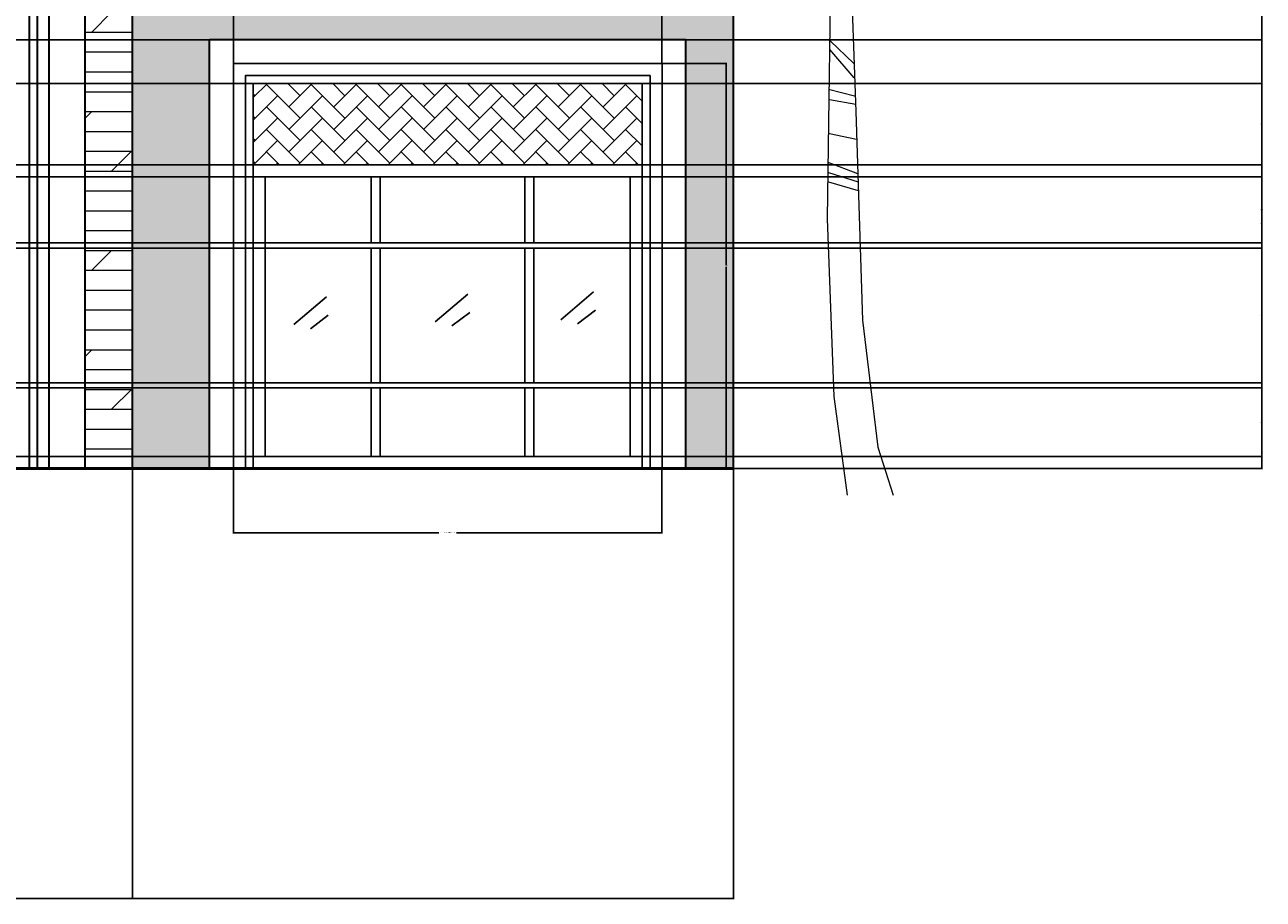
# Model space of a CAD drawing. Units: inches. Extents: x -13 to 630, y -103 to 275.
# Tile 8 of 9: x 318 to 630, y -103 to 117. Entities that reach past the tile are written whole.
import ezdxf

# ---------------------------------------------------------------- set-up
doc = ezdxf.new("R2010")
doc.units = ezdxf.units.IN
doc.header["$MEASUREMENT"] = 0
for name, color, linetype, lineweight in [('A-ANNO-DIMS', 2, 'Continuous', 18), ('A-ELEV', 7, 'Continuous', 35), ('A-ELEV-GRND', 7, 'Continuous', 50), ('A-ELEV-PATT', 8, 'Continuous', 13), ('A-GLAZ', 4, 'Continuous', 25), ('L-PLNT', 3, 'Continuous', 13)]:
    doc.layers.add(name, color=color, linetype=linetype, lineweight=lineweight)
doc.styles.get("Standard").update_dxf_attribs({"font": 'arial.ttf'})
doc.dimstyles.get("Standard").update_dxf_attribs({"dimtxt": 0.18, "dimasz": 0.18, "dimexe": 0.18, "dimexo": 0.0625, "dimgap": 0.09, "dimtad": 0, "dimtih": 1, "dimtoh": 1, "dimdec": 4, "dimzin": 0, "dimdsep": 46, "dimtxsty": 'Standard', "dimcen": 0.09, "dimadec": 0, "dimazin": 0, "dimtfac": 1, "dimtdec": 4, "dimtofl": 0, "dimtmove": 0, "dimatfit": 3, "dimfxl": 1, "dimtolj": 1, "dimtzin": 0, "dimarcsym": 0})

# ---------------------------------------------------------------- blocks, each defined once
blk = doc.blocks.new('*U2')
for p, q in [((-5.567, 196.707), (-4.987, 201.167)), ((-4.407, 195.716), (-3.247, 200.672)), ((-6.727, 197.202), (-11.366, 197.45)), ((-7.5, 199.68), (-7.5, 197.946)), ((-2.474, 193.733), (-1.315, 199.433)), ((-1.121, 190.759), (0.232, 196.955)), ((9.317, 191.255), (10.283, 196.955)), ((11.829, 192.99), (13.182, 197.45)), ((13.956, 194.229), (14.729, 196.955)), ((15.116, 194.477), (17.822, 198.689)), ((18.015, 195.716), (20.914, 198.689)), ((21.301, 196.459), (22.847, 198.441)), ((22.074, 196.707), (23.427, 195.716)), ((23.234, 196.707), (23.62, 197.698)), ((-15.232, 191.255), (-20.644, 193.981)), ((-3.441, 194.477), (-10.013, 195.716)), ((-1.894, 192.494), (-9.24, 193.733)), ((0.038, 188.281), (1.778, 193.981)), ((5.837, 187.786), (7.577, 194.229)), ((14.536, 193.981), (17.242, 191.255)), ((16.082, 194.972), (17.822, 192.494)), ((18.015, 195.468), (18.981, 192.494)), ((19.368, 196.459), (19.948, 193.733)), ((20.914, 196.459), (21.301, 194.972)), ((-29.729, 190.759), (-31.469, 191.255)), ((-30.309, 190.512), (-30.695, 189.025)), ((-25.283, 191.751), (-29.342, 192.246)), ((-28.763, 190.759), (-28.763, 188.281)), ((-26.443, 191.503), (-26.636, 186.051)), ((-20.064, 191.751), (-25.863, 193.238)), ((-23.737, 191.751), (-24.51, 185.06)), ((-21.031, 191.998), (-21.804, 183.325)), ((-17.551, 191.503), (-20.451, 181.343)), ((-14.265, 190.759), (-18.131, 182.086)), ((-9.433, 189.025), (-15.618, 193.238)), ((-0.541, 189.52), (-7.307, 192.494)), ((1.005, 185.803), (2.358, 190.759)), ((4.098, 185.06), (4.678, 190.512)), ((8.544, 190.512), (13.763, 189.52)), ((11.25, 192.494), (15.889, 190.512)), ((-11.753, 189.768), (-15.425, 182.83)), ((-8.08, 188.034), (-12.912, 182.83)), ((-6.147, 186.299), (-9.24, 190.264)), ((-5.76, 190.016), (0.618, 185.308)), ((-5.76, 188.034), (-1.508, 182.582)), ((6.997, 188.529), (12.216, 187.786)), ((9.51, 184.317), (15.502, 188.034)), ((15.695, 186.299), (19.368, 188.777)), ((19.368, 187.29), (26.133, 189.768)), ((23.814, 187.29), (26.907, 181.343)), ((24.78, 187.538), (31.546, 188.777)), ((26.133, 187.29), (29.419, 181.838)), ((28.066, 187.29), (30.966, 182.582)), ((29.999, 186.795), (33.092, 187.29)), ((-4.987, 185.803), (-10.979, 182.086)), ((-2.668, 185.803), (1.198, 181.343)), ((1.005, 182.582), (2.938, 186.547)), ((4.871, 186.051), (10.09, 186.547)), ((4.871, 181.591), (8.544, 184.812)), ((11.25, 184.812), (17.628, 180.352)), ((14.536, 185.803), (19.948, 180.847)), ((17.242, 186.547), (23.041, 180.599)), ((20.721, 187.042), (25.167, 181.343)), ((29.806, 186.795), (32.319, 183.078)), ((32.512, 186.299), (35.218, 186.299)), ((33.479, 186.051), (34.445, 182.83)), ((35.605, 185.556), (37.151, 185.308)), ((35.798, 185.308), (36.958, 181.591)), ((38.118, 184.317), (38.504, 181.838)), ((-3.247, 183.821), (-8.08, 181.838)), ((-1.315, 181.591), (-5.374, 181.095)), ((2.938, 182.582), (6.61, 183.821)), ((5.644, 181.838), (13.569, 178.865)), ((7.77, 183.325), (16.082, 179.856)), ((39.857, 182.83), (40.244, 181.591)), ((-15.618, 179.36), (-20.644, 178.617)), ((-17.358, 178.617), (-13.299, 173.661)), ((-15.038, 179.36), (-10.786, 174.404)), ((-12.332, 180.104), (-9.433, 175.643)), ((-10.206, 180.104), (-8.08, 175.891)), ((-8.273, 180.104), (-6.147, 176.635)), ((-6.34, 179.608), (-4.6, 177.13)), ((-4.021, 179.36), (-2.861, 177.378)), ((-0.348, 180.352), (-1.894, 180.104)), ((4.098, 180.847), (8.35, 179.608)), ((6.224, 178.121), (8.157, 175.148)), ((7.384, 178.369), (10.476, 179.36)), ((8.157, 178.121), (10.476, 172.422)), ((11.829, 177.874), (18.015, 179.113)), ((18.015, 177.13), (26.133, 179.113)), ((-25.09, 175.148), (-28.376, 174.404)), ((-21.031, 177.626), (-24.897, 176.387)), ((-24.317, 175.891), (-18.711, 168.457)), ((-22.191, 176.635), (-16.391, 169.448)), ((-20.064, 177.626), (-15.812, 172.67)), ((-4.214, 175.148), (-14.072, 170.935)), ((-1.701, 176.882), (-8.66, 175.396)), ((-4.6, 174.9), (-4.021, 166.722)), ((-2.668, 176.387), (-2.376, 170.594)), ((-0.928, 176.882), (-1.508, 173.909)), ((2.551, 175.891), (-0.928, 171.431)), ((1.585, 177.13), (0.038, 174.652)), ((1.585, 177.13), (6.61, 176.139)), ((2.938, 175.891), (8.737, 173.413)), ((10.476, 177.874), (12.796, 169.696)), ((13.182, 177.874), (14.729, 166.97)), ((15.889, 177.13), (16.855, 164.492)), ((18.981, 175.891), (19.561, 163.005)), ((20.914, 175.891), (30.966, 176.635)), ((21.688, 175.396), (22.074, 161.518)), ((-28.956, 172.174), (-32.435, 170.192)), ((-27.409, 173.413), (-30.695, 172.67)), ((-27.989, 172.422), (-26.056, 166.227)), ((-26.829, 173.661), (-23.544, 167.218)), ((-25.476, 174.652), (-21.224, 167.466)), ((-8.466, 171.678), (-16.585, 167.713)), ((-6.92, 172.917), (-5.374, 163.253)), ((3.711, 174.404), (-0.541, 167.961)), ((5.257, 171.926), (-0.155, 163.005)), ((4.291, 173.909), (12.216, 168.953)), ((23.814, 174.404), (25.554, 160.279)), ((25.554, 173.661), (33.285, 173.661)), ((26.52, 173.165), (28.066, 159.784)), ((28.839, 172.174), (36.378, 170.687)), ((29.226, 171.926), (30.966, 158.545)), ((-31.082, 169.944), (-32.435, 169.2)), ((-31.662, 168.705), (-31.082, 165.483)), ((-29.922, 170.687), (-27.989, 165.235)), ((-8.853, 170.935), (-7.113, 160.527)), ((7.384, 168.705), (0.812, 157.553)), ((6.417, 170.439), (14.729, 164.492)), ((30.966, 170.687), (38.891, 167.713)), ((32.126, 169.696), (32.512, 158.545)), ((34.058, 168.705), (34.445, 158.545)), ((-32.628, 167.961), (-33.208, 167.961)), ((-32.628, 167.713), (-32.435, 165.979)), ((-12.139, 167.961), (-19.098, 162.014)), ((-12.719, 166.722), (-9.046, 154.828)), ((-10.979, 168.457), (-7.887, 157.801)), ((8.544, 165.979), (16.662, 160.527)), ((35.412, 167.713), (41.404, 164.988)), ((36.378, 166.474), (35.605, 158.792)), ((-14.265, 164.244), (-19.678, 158.049)), ((-14.265, 163.749), (-10.786, 154.828)), ((9.317, 164.244), (2.358, 154.332)), ((10.09, 162.51), (17.435, 157.058)), ((37.731, 165.235), (36.958, 159.288)), ((37.924, 165.235), (41.404, 163.749)), ((38.504, 164.492), (38.504, 159.536)), ((39.664, 163.253), (42.37, 161.766)), ((39.857, 162.757), (39.857, 160.031)), ((-16.005, 160.031), (-19.484, 154.084)), ((-15.618, 160.775), (-12.332, 154.332)), ((10.863, 159.784), (4.484, 152.35)), ((40.824, 161.766), (41.21, 160.031)), ((41.21, 161.518), (42.757, 160.279)), ((-16.585, 158.545), (-13.106, 152.35)), ((11.443, 157.553), (16.855, 154.332)), ((-18.131, 153.589), (-19.484, 151.606)), ((-17.358, 155.819), (-14.845, 151.358)), ((11.829, 155.075), (6.804, 150.119)), ((12.216, 153.093), (16.082, 151.606)), ((-17.938, 152.597), (-16.972, 151.111)), ((12.603, 151.111), (8.544, 148.385)), ((12.603, 149.872), (15.116, 149.128)), ((12.216, 148.137), (10.09, 147.393)), ((12.409, 146.898), (13.763, 146.402)), ((12.409, 145.659), (11.056, 145.659)), ((-4.081, 140.645), (0.753, 138.261)), ((-4.081, 137.547), (0.753, 135.163)), ((-4.081, 129.205), (1.124, 126.821)), ((-4.081, 127.298), (1.31, 123.246)), ((-4.081, 121.578), (1.31, 120.863)), ((-4.267, 114.428), (1.682, 108.708)), ((-4.453, 112.283), (1.682, 105.133)), ((-4.639, 102.273), (1.868, 100.604)), ((-4.453, 99.651), (2.24, 98.459)), ((-4.453, 91.071), (2.426, 89.641)), ((-4.825, 83.921), (2.612, 81.061)), ((-4.639, 81.299), (2.797, 78.916)), ((-4.639, 78.916), (2.797, 76.771))]:
    blk.add_line(p, q)
for points in [[(-2.363, 170.553), (-3.88, 148.505), (-4.988, 69.634), (-3.325, 24.869), (0, 0)], [(-0.116, 162.848), (0.554, 143.532), (2.217, 96.635), (3.88, 44.054), (7.76, 12.079), (11.64, 0)]]:
    blk.add_lwpolyline(points)
for centre, radius, start, end in [((-18.427, 181.448), 19.715, 350.285, 64.11229), ((25.595, 171.567), 25.395, 91.40319, 163.882), ((-21.738, 166.094), 25.899, 27.67115, 112.5305), ((23.687, 155.341), 32.188, 56.19272, 134.3213), ((-9.259, 151.732), 28.386, 68.38311, 147.5322), ((14.394, 148.393), 32.752, 113.7592, 177.4133), ((5.828, 132.718), 45.639, 35.98777, 95.82273), ((-32.8, 147.923), 45.309, 356.1943, 41.37848)]:
    blk.add_arc(centre, radius, start, end)
blk = doc.blocks.new('WIN-GROUND')
for points in [[(0, 0), (0, 102), (108, 102), (108, 0)], [(3, 0), (3, 99), (105, 99), (105, 0)], [(5, 0), (5, 97), (103, 97), (103, 0)], [(34.74, 56.82), (34.74, 73.49), (37, 73.49), (37, 56.82)], [(73.43, 56.82), (73.43, 73.49), (75.7, 73.49), (75.7, 56.82)], [(34.74, 55.51), (8, 55.51), (8, 56.82), (34.74, 56.82)], [(37, 56.82), (73.43, 56.82)], [(75.7, 56.82), (100, 56.82), (100, 55.51), (75.7, 55.51)], [(34.74, 21.58), (34.74, 55.51)], [(37, 55.51), (37, 21.58)], [(73.43, 55.51), (37, 55.51)], [(73.43, 21.58), (73.43, 55.51)], [(75.7, 55.51), (75.7, 21.58)], [(34.74, 20.27), (8, 20.27), (8, 21.58), (34.74, 21.58)], [(37, 20.27), (37, 3), (34.74, 3), (34.74, 20.27)], [(37, 21.58), (73.43, 21.58)], [(73.43, 20.27), (37, 20.27)], [(75.7, 20.27), (75.7, 3), (73.43, 3), (73.43, 20.27)], [(75.7, 21.58), (100, 21.58), (100, 20.27), (75.7, 20.27)]]:
    blk.add_lwpolyline(points)
for points in [[(5, 97), (103, 97), (103, 76.49), (5, 76.49)], [(5, 76.49), (103, 76.49), (103, 0), (5, 0)], [(8, 73.49), (100, 73.49), (100, 3), (8, 3)]]:
    blk.add_lwpolyline(points, close=True)
blk = doc.blocks.new('GLAZ-MARK')
for p, q in [((0, 1.02), (8.26, 8.03)), ((4.19, 0), (8.71, 3.39))]:
    blk.add_line(p, q)
blk = doc.blocks.new('*D5')
at = {"layer": 'A-ANNO-DIMS', "color": 0, "lineweight": -2, "transparency": 16777216}
for p, q in [((370.71, 5.02), (370.71, -11.3)), ((478.71, 5.02), (478.71, -11.3)), ((370.89, -11.12), (422.47, -11.12)), ((478.53, -11.12), (426.96, -11.12))]:
    blk.add_line(p, q, dxfattribs=at)
at = {"layer": 'A-ANNO-DIMS', "color": 0, "transparency": 16777216}
for points in [[(370.89, -11.09), (370.89, -11.15), (370.71, -11.12)], [(478.53, -11.09), (478.53, -11.15), (478.71, -11.12)]]:
    blk.add_solid(points, dxfattribs=at)
at = {"layer": 'Defpoints', "color": 0, "transparency": 16777216}
for p in [(370.71, 5.08), (478.71, 5.08), (478.71, -11.12)]:
    blk.add_point(p, dxfattribs=at)
at = {"layer": 'A-ANNO-DIMS', "color": 0, "transparency": 16777216, "insert": (424.71, -11.12), "char_height": 0.18, "attachment_point": 5}
blk.add_mtext('\\A1;GROUND FLOOR WINDOW 108 TYP.', dxfattribs=at)
blk = doc.blocks.new('*D6')
at = {"layer": 'A-ANNO-DIMS', "color": 0, "lineweight": -2, "transparency": 16777216}
for p, q in [((478.77, 107.08), (495.09, 107.08)), ((494.91, 106.9), (494.91, 56.26)), ((494.91, 5.26), (494.91, 55.9)), ((478.77, 5.08), (495.09, 5.08))]:
    blk.add_line(p, q, dxfattribs=at)
at = {"layer": 'A-ANNO-DIMS', "color": 0, "transparency": 16777216}
for points in [[(494.88, 106.9), (494.94, 106.9), (494.91, 107.08)], [(494.88, 5.26), (494.94, 5.26), (494.91, 5.08)]]:
    blk.add_solid(points, dxfattribs=at)
at = {"layer": 'Defpoints', "color": 0, "transparency": 16777216}
for p in [(478.71, 107.08), (494.91, 107.08), (478.71, 5.08)]:
    blk.add_point(p, dxfattribs=at)
at = {"layer": 'A-ANNO-DIMS', "color": 0, "transparency": 16777216, "insert": (494.91, 56.08), "char_height": 0.18, "attachment_point": 5}
blk.add_mtext('\\A1;102 TYP.', dxfattribs=at)
blk = doc.blocks.new('*D9')
at = {"layer": 'A-ANNO-DIMS', "color": 0, "lineweight": -2, "transparency": 16777216}
for p, q in [((345.31, 5.14), (345.31, 275.01)), ((345.49, 274.83), (357.54, 274.83)), ((370.53, 274.83), (358.47, 274.83)), ((370.71, 5.14), (370.71, 275.01))]:
    blk.add_line(p, q, dxfattribs=at)
at = {"layer": 'A-ANNO-DIMS', "color": 0, "transparency": 16777216}
for points in [[(345.49, 274.86), (345.49, 274.8), (345.31, 274.83)], [(370.53, 274.86), (370.53, 274.8), (370.71, 274.83)]]:
    blk.add_solid(points, dxfattribs=at)
at = {"layer": 'Defpoints', "color": 0, "transparency": 16777216}
for p in [(370.71, 274.83), (345.31, 5.08), (370.71, 5.08)]:
    blk.add_point(p, dxfattribs=at)
at = {"layer": 'A-ANNO-DIMS', "color": 0, "transparency": 16777216, "insert": (358.01, 274.83), "char_height": 0.18, "attachment_point": 5}
blk.add_mtext('\\A1;25.406', dxfattribs=at)
blk = doc.blocks.new('*D10')
at = {"layer": 'A-ANNO-DIMS', "color": 0, "lineweight": -2, "transparency": 16777216}
for p, q in [((478.71, 107.14), (478.71, 275.01)), ((478.89, 274.83), (487.5, 274.83)), ((496.53, 274.83), (487.92, 274.83)), ((496.71, 125.14), (496.71, 275.01))]:
    blk.add_line(p, q, dxfattribs=at)
at = {"layer": 'A-ANNO-DIMS', "color": 0, "transparency": 16777216}
for points in [[(478.89, 274.86), (478.89, 274.8), (478.71, 274.83)], [(496.53, 274.86), (496.53, 274.8), (496.71, 274.83)]]:
    blk.add_solid(points, dxfattribs=at)
at = {"layer": 'Defpoints', "color": 0, "transparency": 16777216}
for p in [(496.71, 274.83), (496.71, 125.08), (478.71, 107.08)]:
    blk.add_point(p, dxfattribs=at)
at = {"layer": 'A-ANNO-DIMS', "color": 0, "transparency": 16777216, "insert": (487.71, 274.83), "char_height": 0.18, "attachment_point": 5}
blk.add_mtext('\\A1;18', dxfattribs=at)
blk = doc.blocks.new('*D11')
at = {"layer": 'A-ANNO-DIMS', "color": 0, "lineweight": -2, "transparency": 16777216}
for p, q in [((16.71, 5.02), (16.71, -103.45)), ((496.71, 5.02), (496.71, -103.45)), ((16.89, -103.27), (256.42, -103.27)), ((496.53, -103.27), (257, -103.27))]:
    blk.add_line(p, q, dxfattribs=at)
at = {"layer": 'A-ANNO-DIMS', "color": 0, "transparency": 16777216}
for points in [[(16.89, -103.24), (16.89, -103.3), (16.71, -103.27)], [(496.53, -103.24), (496.53, -103.3), (496.71, -103.27)]]:
    blk.add_solid(points, dxfattribs=at)
at = {"layer": 'Defpoints', "color": 0, "transparency": 16777216}
for p in [(16.71, 5.08), (496.71, 5.08), (496.71, -103.27)]:
    blk.add_point(p, dxfattribs=at)
at = {"layer": 'A-ANNO-DIMS', "color": 0, "transparency": 16777216, "insert": (256.71, -103.27), "char_height": 0.18, "attachment_point": 5}
blk.add_mtext('\\A1;480', dxfattribs=at)
blk = doc.blocks.new('*D13')
at = {"layer": 'A-ANNO-DIMS', "color": 0, "lineweight": -2, "transparency": 16777216}
for p, q in [((345.37, 245.08), (630.03, 245.08)), ((629.85, 244.9), (629.85, 125.26)), ((629.85, 5.26), (629.85, 124.9)), ((496.77, 5.08), (630.03, 5.08))]:
    blk.add_line(p, q, dxfattribs=at)
at = {"layer": 'A-ANNO-DIMS', "color": 0, "transparency": 16777216}
for points in [[(629.82, 244.9), (629.88, 244.9), (629.85, 245.08)], [(629.82, 5.26), (629.88, 5.26), (629.85, 5.08)]]:
    blk.add_solid(points, dxfattribs=at)
at = {"layer": 'Defpoints', "color": 0, "transparency": 16777216}
for p in [(345.31, 245.08), (629.85, 245.08), (496.71, 5.08)]:
    blk.add_point(p, dxfattribs=at)
at = {"layer": 'A-ANNO-DIMS', "color": 0, "transparency": 16777216, "insert": (629.85, 125.08), "char_height": 0.18, "attachment_point": 5}
blk.add_mtext('\\A1;240', dxfattribs=at)
blk = doc.blocks.new('*D26')
at = {"layer": 'A-ANNO-DIMS', "color": 0, "lineweight": -2, "transparency": 16777216}
for p, q in [((302.53, 5.02), (302.53, -103.45)), ((345.31, 5.02), (345.31, -103.45)), ((302.71, -103.27), (323.52, -103.27)), ((345.13, -103.27), (324.31, -103.27))]:
    blk.add_line(p, q, dxfattribs=at)
at = {"layer": 'A-ANNO-DIMS', "color": 0, "transparency": 16777216}
for points in [[(302.71, -103.24), (302.71, -103.3), (302.53, -103.27)], [(345.13, -103.24), (345.13, -103.3), (345.31, -103.27)]]:
    blk.add_solid(points, dxfattribs=at)
at = {"layer": 'Defpoints', "color": 0, "transparency": 16777216}
for p in [(302.53, 5.08), (345.31, 5.08), (345.31, -103.27)]:
    blk.add_point(p, dxfattribs=at)
at = {"layer": 'A-ANNO-DIMS', "color": 0, "transparency": 16777216, "insert": (323.92, -103.27), "char_height": 0.18, "attachment_point": 5}
blk.add_mtext('\\A1;42.78', dxfattribs=at)
blk = doc.blocks.new('*D28')
at = {"layer": 'A-ANNO-DIMS', "color": 0, "lineweight": -2, "transparency": 16777216}
for p, q in [((302.59, 128.66), (630.03, 128.66)), ((629.85, 128.48), (629.85, 67.05)), ((629.85, 5.26), (629.85, 66.69)), ((302.59, 5.08), (630.03, 5.08))]:
    blk.add_line(p, q, dxfattribs=at)
at = {"layer": 'A-ANNO-DIMS', "color": 0, "transparency": 16777216}
for points in [[(629.82, 128.48), (629.88, 128.48), (629.85, 128.66)], [(629.82, 5.26), (629.88, 5.26), (629.85, 5.08)]]:
    blk.add_solid(points, dxfattribs=at)
at = {"layer": 'Defpoints', "color": 0, "transparency": 16777216}
for p in [(302.53, 128.66), (629.85, 128.66), (302.53, 5.08)]:
    blk.add_point(p, dxfattribs=at)
at = {"layer": 'A-ANNO-DIMS', "color": 0, "transparency": 16777216, "insert": (629.85, 66.87), "char_height": 0.18, "attachment_point": 5}
blk.add_mtext('\\A1;123.57', dxfattribs=at)
blk = doc.blocks.new('*D78')
at = {"layer": 'A-ANNO-DIMS', "color": 0, "lineweight": -2, "transparency": 16777216}
for p, q in [((134.77, 8.08), (630.03, 8.08)), ((629.85, 7.9), (629.85, 6.76)), ((629.85, 5.26), (629.85, 6.4)), ((137.77, 5.08), (630.03, 5.08))]:
    blk.add_line(p, q, dxfattribs=at)
at = {"layer": 'A-ANNO-DIMS', "color": 0, "transparency": 16777216}
for points in [[(629.82, 7.9), (629.88, 7.9), (629.85, 8.08)], [(629.82, 5.26), (629.88, 5.26), (629.85, 5.08)]]:
    blk.add_solid(points, dxfattribs=at)
at = {"layer": 'Defpoints', "color": 0, "transparency": 16777216}
for p in [(134.71, 8.08), (629.85, 8.08), (137.71, 5.08)]:
    blk.add_point(p, dxfattribs=at)
at = {"layer": 'A-ANNO-DIMS', "color": 0, "transparency": 16777216, "insert": (629.85, 6.58), "char_height": 0.18, "attachment_point": 5}
blk.add_mtext('\\A1;3', dxfattribs=at)
blk = doc.blocks.new('*D79')
at = {"layer": 'A-ANNO-DIMS', "color": 0, "lineweight": -2, "transparency": 16777216}
for p, q in [((134.77, 25.35), (630.03, 25.35)), ((629.85, 25.17), (629.85, 16.9)), ((629.85, 8.26), (629.85, 16.53)), ((134.77, 8.08), (630.03, 8.08))]:
    blk.add_line(p, q, dxfattribs=at)
at = {"layer": 'A-ANNO-DIMS', "color": 0, "transparency": 16777216}
for points in [[(629.82, 25.17), (629.88, 25.17), (629.85, 25.35)], [(629.82, 8.26), (629.88, 8.26), (629.85, 8.08)]]:
    blk.add_solid(points, dxfattribs=at)
at = {"layer": 'Defpoints', "color": 0, "transparency": 16777216}
for p in [(134.71, 25.35), (629.85, 25.35), (134.71, 8.08)]:
    blk.add_point(p, dxfattribs=at)
at = {"layer": 'A-ANNO-DIMS', "color": 0, "transparency": 16777216, "insert": (629.85, 16.72), "char_height": 0.18, "attachment_point": 5}
blk.add_mtext('\\A1;17.27', dxfattribs=at)
blk = doc.blocks.new('*D80')
at = {"layer": 'A-ANNO-DIMS', "color": 0, "lineweight": -2, "transparency": 16777216}
for p, q in [((134.77, 26.66), (630.03, 26.66)), ((134.77, 25.35), (630.03, 25.35)), ((629.85, 26.48), (629.85, 26.19)), ((629.85, 25.53), (629.85, 25.82))]:
    blk.add_line(p, q, dxfattribs=at)
at = {"layer": 'A-ANNO-DIMS', "color": 0, "transparency": 16777216}
for points in [[(629.82, 26.48), (629.88, 26.48), (629.85, 26.66)], [(629.82, 25.53), (629.88, 25.53), (629.85, 25.35)]]:
    blk.add_solid(points, dxfattribs=at)
at = {"layer": 'Defpoints', "color": 0, "transparency": 16777216}
for p in [(134.71, 26.66), (134.71, 25.35), (629.85, 26.66)]:
    blk.add_point(p, dxfattribs=at)
at = {"layer": 'A-ANNO-DIMS', "color": 0, "transparency": 16777216, "insert": (629.85, 26), "char_height": 0.18, "attachment_point": 5}
blk.add_mtext('\\A1;1.31', dxfattribs=at)
blk = doc.blocks.new('*D81')
at = {"layer": 'A-ANNO-DIMS', "color": 0, "lineweight": -2, "transparency": 16777216}
for p, q in [((134.77, 60.6), (630.03, 60.6)), ((629.85, 60.42), (629.85, 43.81)), ((629.85, 26.84), (629.85, 43.44)), ((134.77, 26.66), (630.03, 26.66))]:
    blk.add_line(p, q, dxfattribs=at)
at = {"layer": 'A-ANNO-DIMS', "color": 0, "transparency": 16777216}
for points in [[(629.82, 60.42), (629.88, 60.42), (629.85, 60.6)], [(629.82, 26.84), (629.88, 26.84), (629.85, 26.66)]]:
    blk.add_solid(points, dxfattribs=at)
at = {"layer": 'Defpoints', "color": 0, "transparency": 16777216}
for p in [(134.71, 60.6), (629.85, 60.6), (134.71, 26.66)]:
    blk.add_point(p, dxfattribs=at)
at = {"layer": 'A-ANNO-DIMS', "color": 0, "transparency": 16777216, "insert": (629.85, 43.63), "char_height": 0.18, "attachment_point": 5}
blk.add_mtext('\\A1;33.94', dxfattribs=at)
blk = doc.blocks.new('*D82')
at = {"layer": 'A-ANNO-DIMS', "color": 0, "lineweight": -2, "transparency": 16777216}
for p, q in [((134.77, 61.9), (630.03, 61.9)), ((134.77, 60.6), (630.03, 60.6)), ((629.85, 61.72), (629.85, 61.43)), ((629.85, 60.78), (629.85, 61.07))]:
    blk.add_line(p, q, dxfattribs=at)
at = {"layer": 'A-ANNO-DIMS', "color": 0, "transparency": 16777216}
for points in [[(629.82, 61.72), (629.88, 61.72), (629.85, 61.9)], [(629.82, 60.78), (629.88, 60.78), (629.85, 60.6)]]:
    blk.add_solid(points, dxfattribs=at)
at = {"layer": 'Defpoints', "color": 0, "transparency": 16777216}
for p in [(134.71, 61.9), (134.71, 60.6), (629.85, 61.9)]:
    blk.add_point(p, dxfattribs=at)
at = {"layer": 'A-ANNO-DIMS', "color": 0, "transparency": 16777216, "insert": (629.85, 61.25), "char_height": 0.18, "attachment_point": 5}
blk.add_mtext('\\A1;1.31', dxfattribs=at)
blk = doc.blocks.new('*D83')
at = {"layer": 'A-ANNO-DIMS', "color": 0, "lineweight": -2, "transparency": 16777216}
for p, q in [((134.77, 78.57), (630.03, 78.57)), ((629.85, 78.39), (629.85, 70.42)), ((629.85, 62.08), (629.85, 70.05)), ((134.77, 61.9), (630.03, 61.9))]:
    blk.add_line(p, q, dxfattribs=at)
at = {"layer": 'A-ANNO-DIMS', "color": 0, "transparency": 16777216}
for points in [[(629.82, 78.39), (629.88, 78.39), (629.85, 78.57)], [(629.82, 62.08), (629.88, 62.08), (629.85, 61.9)]]:
    blk.add_solid(points, dxfattribs=at)
at = {"layer": 'Defpoints', "color": 0, "transparency": 16777216}
for p in [(134.71, 78.57), (629.85, 78.57), (134.71, 61.9)]:
    blk.add_point(p, dxfattribs=at)
at = {"layer": 'A-ANNO-DIMS', "color": 0, "transparency": 16777216, "insert": (629.85, 70.24), "char_height": 0.18, "attachment_point": 5}
blk.add_mtext('\\A1;16.67', dxfattribs=at)
blk = doc.blocks.new('*D84')
at = {"layer": 'A-ANNO-DIMS', "color": 0, "lineweight": -2, "transparency": 16777216}
for p, q in [((137.77, 81.57), (630.03, 81.57)), ((629.85, 81.39), (629.85, 80.25)), ((134.77, 78.57), (630.03, 78.57)), ((629.85, 78.75), (629.85, 79.89))]:
    blk.add_line(p, q, dxfattribs=at)
at = {"layer": 'A-ANNO-DIMS', "color": 0, "transparency": 16777216}
for points in [[(629.82, 81.39), (629.88, 81.39), (629.85, 81.57)], [(629.82, 78.75), (629.88, 78.75), (629.85, 78.57)]]:
    blk.add_solid(points, dxfattribs=at)
at = {"layer": 'Defpoints', "color": 0, "transparency": 16777216}
for p in [(137.71, 81.57), (629.85, 81.57), (134.71, 78.57)]:
    blk.add_point(p, dxfattribs=at)
at = {"layer": 'A-ANNO-DIMS', "color": 0, "transparency": 16777216, "insert": (629.85, 80.07), "char_height": 0.18, "attachment_point": 5}
blk.add_mtext('\\A1;3', dxfattribs=at)
blk = doc.blocks.new('*D85')
at = {"layer": 'A-ANNO-DIMS', "color": 0, "lineweight": -2, "transparency": 16777216}
for p, q in [((137.77, 102.08), (630.03, 102.08)), ((629.85, 101.9), (629.85, 92.01)), ((629.85, 81.75), (629.85, 91.64)), ((137.77, 81.57), (630.03, 81.57))]:
    blk.add_line(p, q, dxfattribs=at)
at = {"layer": 'A-ANNO-DIMS', "color": 0, "transparency": 16777216}
for points in [[(629.82, 101.9), (629.88, 101.9), (629.85, 102.08)], [(629.82, 81.75), (629.88, 81.75), (629.85, 81.57)]]:
    blk.add_solid(points, dxfattribs=at)
at = {"layer": 'Defpoints', "color": 0, "transparency": 16777216}
for p in [(137.71, 102.08), (629.85, 102.08), (137.71, 81.57)]:
    blk.add_point(p, dxfattribs=at)
at = {"layer": 'A-ANNO-DIMS', "color": 0, "transparency": 16777216, "insert": (629.85, 91.83), "char_height": 0.18, "attachment_point": 5}
blk.add_mtext('\\A1;20.51', dxfattribs=at)
blk = doc.blocks.new('*D86')
at = {"layer": 'A-ANNO-DIMS', "color": 0, "lineweight": -2, "transparency": 16777216}
for p, q in [((148.77, 113.08), (630.03, 113.08)), ((629.85, 112.9), (629.85, 107.76)), ((629.85, 102.26), (629.85, 107.4)), ((137.77, 102.08), (630.03, 102.08))]:
    blk.add_line(p, q, dxfattribs=at)
at = {"layer": 'A-ANNO-DIMS', "color": 0, "transparency": 16777216}
for points in [[(629.82, 112.9), (629.88, 112.9), (629.85, 113.08)], [(629.82, 102.26), (629.88, 102.26), (629.85, 102.08)]]:
    blk.add_solid(points, dxfattribs=at)
at = {"layer": 'Defpoints', "color": 0, "transparency": 16777216}
for p in [(148.71, 113.08), (629.85, 113.08), (137.71, 102.08)]:
    blk.add_point(p, dxfattribs=at)
at = {"layer": 'A-ANNO-DIMS', "color": 0, "transparency": 16777216, "insert": (629.85, 107.58), "char_height": 0.18, "attachment_point": 5}
blk.add_mtext('\\A1;11', dxfattribs=at)

msp = doc.modelspace()

# ---------------------------------------------------------------- hatches: boundary and pattern name
at = {"layer": 'A-ELEV-PATT', "transparency": 33554541}
h = msp.add_hatch(dxfattribs=at)
h.set_pattern_fill('DOLMIT', color=256, scale=20)
h.paths.add_polyline_path([(345.3061, 245.0808), (164.8443, 245.0808), (164.8443, 5.0808), (176.8443, 5.0808), (176.8443, 233.0808), (333.3061, 233.0808), (333.3061, 5.0808), (345.3061, 5.0808)])
at = {"layer": 'A-ELEV-PATT'}
h = msp.add_hatch(dxfattribs=at)
h.set_pattern_fill('BRSTONE', color=256, scale=20)
h.paths.add_polyline_path([(120.6641, 172.7854), (64.9953, 172.7854, 0.41421356), (54.9953, 162.7854), (54.9953, 125.0808), (59.9953, 125.0808), (59.9953, 162.7854, -0.41421356), (64.9953, 167.7854), (120.6641, 167.7854, -0.41421356), (125.6641, 162.7854), (125.6641, 125.0808), (130.6641, 125.0808), (130.6641, 162.7854, 0.41421356)])
h.paths.add_polyline_path([(439.5513, 172.7854), (383.8825, 172.7854, 0.41421356), (373.8825, 162.7854), (373.8825, 125.0808), (378.8825, 125.0808), (378.8825, 162.7854, -0.41421356), (383.8825, 167.7854), (439.5513, 167.7854, -0.41421356), (444.5513, 162.7854), (444.5513, 125.0808), (449.5513, 125.0808), (449.5513, 162.7854, 0.41421356)])
h.paths.add_polyline_path([(364.7117, 113.0808), (484.7117, 113.0808), (484.7117, 5.0808), (496.7117, 5.0808), (496.7117, 125.0808), (345.3061, 125.0808), (345.3061, 5.0808), (364.7117, 5.0808)])
h.paths.add_polyline_path([(164.8443, 125.0808), (28.7117, 125.0808), (16.7117, 125.0808), (16.7117, 5.0808), (28.7117, 5.0808), (28.7117, 113.0808), (148.7117, 113.0808), (148.7117, 5.0808), (164.8443, 5.0808)])
h.paths.add_polyline_path([(95.1171, 223.9392), (83.8622, 223.9392), (83.8622, 206.5279), (95.1171, 206.5279)])
h.paths.add_polyline_path([(54.9212, 223.9392), (40.7186, 223.9392), (40.7186, 206.5279), (54.9212, 206.5279)])
h.paths.add_polyline_path([(463.828, 223.9392), (449.6254, 223.9392), (449.6254, 206.5279), (463.828, 206.5279)])
h.paths.add_polyline_path([(420.6843, 223.9392), (409.4295, 223.9392), (409.4295, 206.5279), (420.6843, 206.5279)])
h = msp.add_hatch(dxfattribs=at)
h.set_pattern_fill('AR-HBONE', color=256)
h.paths.add_polyline_path([(137.7117, 102.0808), (39.7117, 102.0808), (39.7117, 81.5713), (137.7117, 81.5713)])
h.paths.add_polyline_path([(473.7117, 102.0808), (375.7117, 102.0808), (375.7117, 81.5713), (473.7117, 81.5713)])

# ---------------------------------------------------------------- linework, layer by layer
at = {"layer": 'A-ELEV'}
for p, q in [((484.7117, 113.0808), (364.7117, 113.0808)), ((364.7117, 5.0808), (364.7117, 113.0808)), ((484.7117, 5.0808), (484.7117, 113.0808)), ((164.8443, 5.0808), (345.3061, 5.0808))]:
    msp.add_line(p, q, dxfattribs=at)
for points in [[(345.3061, 5.0808), (345.3061, 245.0808), (164.8443, 245.0808), (164.8443, 5.0808)], [(333.3061, 5.0808), (333.3061, 233.0808), (176.8443, 233.0808), (176.8443, 5.0808)], [(324.3061, 5.0808), (324.3061, 224.0808), (185.8443, 224.0808), (185.8443, 5.0808)], [(321.3061, 5.0808), (321.3061, 221.0808), (188.8443, 221.0808), (188.8443, 5.0808)], [(319.3061, 5.0808), (319.3061, 219.0808), (190.8443, 219.0808), (190.8443, 5.0808)], [(496.7117, 5.0808), (496.7117, 125.0808), (345.3061, 125.0808)]]:
    msp.add_lwpolyline(points, dxfattribs=at)
at = {"layer": 'A-ELEV-GRND'}
msp.add_line((16.7117, 5.0808), (496.7117, 5.0808), dxfattribs=at)

# ---------------------------------------------------------------- block references
at = {"layer": 'A-GLAZ'}
for name, p in [('WIN-GROUND', (370.712, 5.081)), ('GLAZ-MARK', (385.9023, 40.2964)), ('GLAZ-MARK', (421.5495, 40.9769)), ('GLAZ-MARK', (453.2234, 41.544))]:
    msp.add_blockref(name, p, dxfattribs=at)
at = {"layer": 'L-PLNT'}
msp.add_blockref('*U2', (525.3348, -1.6376), dxfattribs=at)

# ---------------------------------------------------------------- dimensions: what is measured, and where the dimension line sits
at = {"layer": 'A-ANNO-DIMS'}
for base, p1, p2, override, picture, middle in [((370.7117, 274.8308), (345.3061, 5.0808), (370.7117, 5.0808), {"dimdec": 3, "dimlfac": 1, "dimrnd": 0, "dimzin": 0, "dimdsep": 46, "dimlunit": 2}, '*D9', (358.0089, 274.8308)), ((496.7117, 274.8308), (478.7117, 107.0808), (496.7117, 125.0808), {"dimdec": 0, "dimlfac": 1, "dimrnd": 0, "dimzin": 0, "dimdsep": 46, "dimlunit": 2}, '*D10', (487.7117, 274.8308)), ((496.7117, -103.2746), (16.7117, 5.0808), (496.7117, 5.0808), {"dimdec": 0, "dimlfac": 1, "dimrnd": 0, "dimzin": 0, "dimdsep": 46, "dimlunit": 2}, '*D11', (256.7117, -103.2746)), ((345.3061, -103.2746), (302.5258, 5.0808), (345.3061, 5.0808), {"dimdec": 2, "dimlfac": 1, "dimrnd": 0, "dimzin": 0, "dimdsep": 46, "dimlunit": 2}, '*D26', (323.9159, -103.2746))]:
    dim = msp.add_linear_dim(base=base, p1=p1, p2=p2, dimstyle='Standard', override=override, dxfattribs=at)
    dim.commit()
    dim.dimension.update_dxf_attribs({"geometry": picture, "text_midpoint": middle})
for base, p1, p2, override, picture, middle in [((629.8508, 245.0808), (496.7117, 5.0808), (345.3061, 245.0808), {"dimdec": 0, "dimlfac": 1, "dimrnd": 0, "dimzin": 0, "dimdsep": 46, "dimlunit": 2}, '*D13', (629.8508, 125.0808)), ((629.8508, 128.6551), (302.5258, 5.0808), (302.5258, 128.6551), {"dimdec": 2, "dimlfac": 1, "dimrnd": 0, "dimzin": 0, "dimdsep": 46, "dimlunit": 2}, '*D28', (629.8508, 66.868)), ((629.8508, 113.0808), (137.7117, 102.0808), (148.7117, 113.0808), {"dimdec": 0, "dimlfac": 1, "dimrnd": 0, "dimzin": 0, "dimdsep": 46, "dimlunit": 2}, '*D86', (629.8508, 107.5808)), ((629.8508, 102.0808), (137.7117, 81.5713), (137.7117, 102.0808), {"dimdec": 2, "dimlfac": 1, "dimrnd": 0, "dimzin": 0, "dimdsep": 46, "dimlunit": 2}, '*D85', (629.8508, 91.826)), ((629.8508, 81.5713), (134.7117, 78.5713), (137.7117, 81.5713), {"dimdec": 0, "dimlfac": 1, "dimrnd": 0, "dimzin": 0, "dimdsep": 46, "dimlunit": 2}, '*D84', (629.8508, 80.0713)), ((629.8508, 78.5713), (134.7117, 61.902), (134.7117, 78.5713), {"dimdec": 2, "dimlfac": 1, "dimrnd": 0, "dimzin": 0, "dimdsep": 46, "dimlunit": 2}, '*D83', (629.8508, 70.2366)), ((629.8508, 61.902), (134.7117, 60.5952), (134.7117, 61.902), {"dimdec": 2, "dimlfac": 1, "dimrnd": 0, "dimzin": 0, "dimdsep": 46, "dimlunit": 2}, '*D82', (629.8508, 61.2486)), ((629.8508, 60.5952), (134.7117, 26.6567), (134.7117, 60.5952), {"dimdec": 2, "dimlfac": 1, "dimrnd": 0, "dimzin": 0, "dimdsep": 46, "dimlunit": 2}, '*D81', (629.8508, 43.6259)), ((629.8508, 26.6567), (134.7117, 25.3499), (134.7117, 26.6567), {"dimdec": 2, "dimlfac": 1, "dimrnd": 0, "dimzin": 0, "dimdsep": 46, "dimlunit": 2}, '*D80', (629.8508, 26.0033)), ((629.8508, 25.3499), (134.7117, 8.0808), (134.7117, 25.3499), {"dimdec": 2, "dimlfac": 1, "dimrnd": 0, "dimzin": 0, "dimdsep": 46, "dimlunit": 2}, '*D79', (629.8508, 16.7154)), ((629.8508, 8.0808), (137.7117, 5.0808), (134.7117, 8.0808), {"dimdec": 0, "dimlfac": 1, "dimrnd": 0, "dimzin": 0, "dimdsep": 46, "dimlunit": 2}, '*D78', (629.8508, 6.5808))]:
    dim = msp.add_linear_dim(base=base, p1=p1, p2=p2, angle=90, dimstyle='Standard', override=override, dxfattribs=at)
    dim.commit()
    dim.dimension.update_dxf_attribs({"geometry": picture, "text_midpoint": middle})
dim = msp.add_linear_dim(base=(494.9117, 107.0808), p1=(478.7117, 5.0808), p2=(478.7117, 107.0808), angle=90, text='<> TYP.', dimstyle='Standard', override={"dimdec": 0, "dimlfac": 1, "dimrnd": 0, "dimzin": 0, "dimdsep": 46, "dimlunit": 2}, dxfattribs=at)
dim.commit()
dim.dimension.update_dxf_attribs({"geometry": '*D6', "text_midpoint": (494.9117, 56.0808)})
dim = msp.add_linear_dim(base=(478.7117, -11.1192), p1=(370.7117, 5.0808), p2=(478.7117, 5.0808), text='GROUND FLOOR WINDOW <> TYP.', dimstyle='Standard', override={"dimdec": 0, "dimlfac": 1, "dimrnd": 0, "dimzin": 0, "dimdsep": 46, "dimlunit": 2}, dxfattribs=at)
dim.commit()
dim.dimension.update_dxf_attribs({"geometry": '*D5', "text_midpoint": (424.7117, -11.1192)})

doc.saveas('drawing.dxf')
